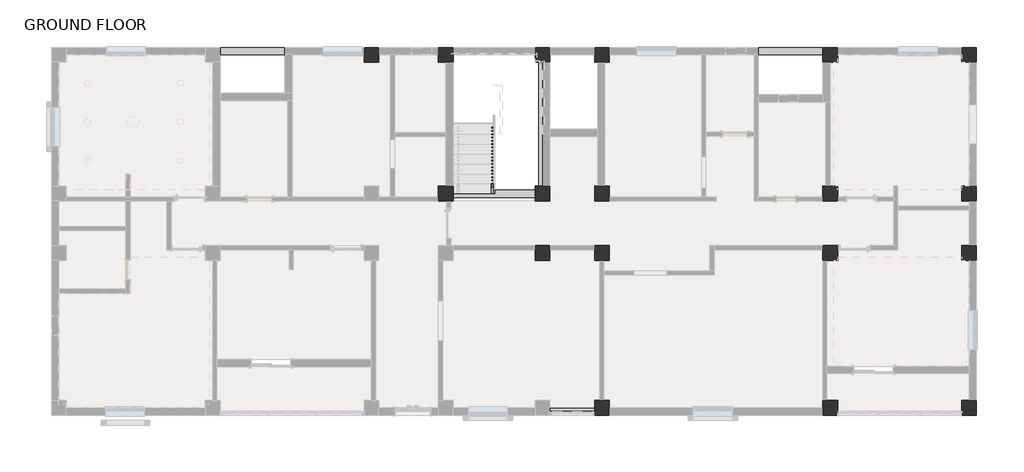
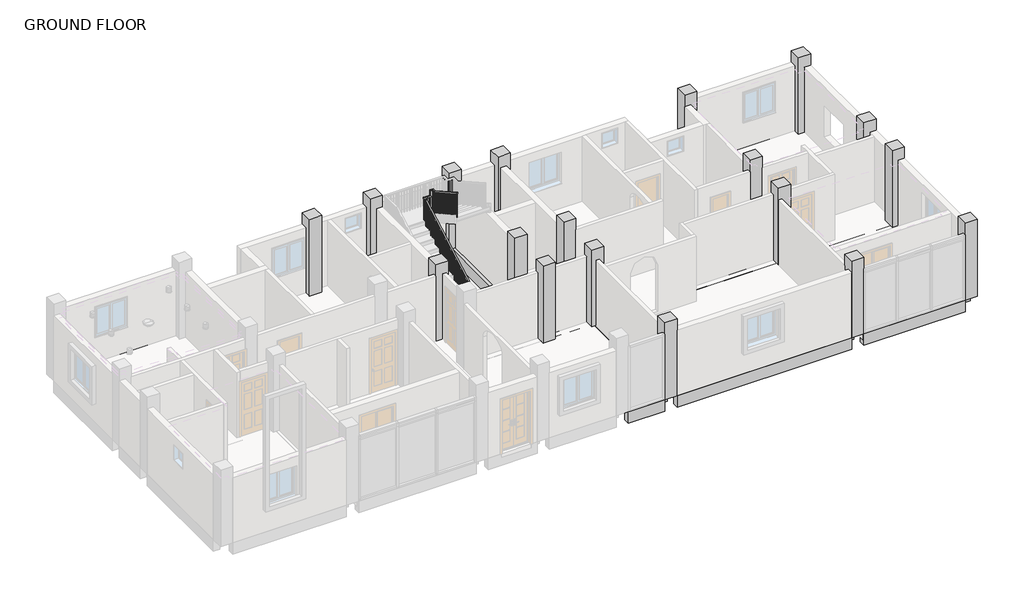
# One storey, part 4 of 5: 31 beams, 18 columns, 1 railing.
"""IFC4 building model written with IfcOpenShell, lengths in millimetres."""

from ifc_helpers import new_model, si_unit, frame, origin, place, context, project, spatial, polyline, outline, extrude, faceted_brep, element, save

model = new_model("IFC4")

# Units and contexts
model_context = context("Model", 3, world=origin())
ifc_project = project(units=[si_unit("LENGTHUNIT", "METRE", prefix="MILLI")], contexts=[model_context])

# Site, building, storey
site = spatial("IfcSite", under=ifc_project)
building = spatial("IfcBuilding", under=site)
storey = spatial("IfcBuildingStorey", under=building, Name="GROUND FLOOR", Elevation=304.8)

# Beams
placement = place(None, origin())
element("IfcBeam", 1, ObjectType="Concrete-Rectangular Beam : 9\" X 18\" BEAM", at=placement, inside=storey, context=model_context, shape_type="SweptSolid", body=[
    extrude(outline(polyline([(1310.3916602, -10887.8679047), (1310.3916602, -11116.4679047), (-61.2083398, -11116.4679047), (-61.2083398, -10887.8679047), (1310.3916602, -10887.8679047)])), frame((0.0, 0.0, -152.4), z_axis=(0.0, 0.0, 1.0), x_axis=(1.0, 0.0, 0.0)), (0.0, 0.0, 1.0), 457.2),
])
element("IfcBeam", 2, ObjectType="Concrete-Rectangular Beam : 9\" X 18\" BEAM", at=placement, inside=storey, context=model_context, shape_type="Brep", body=[
    faceted_brep([(1424.6916602, -6358.3794704, 304.8), (1424.6916602, -10659.2679047, 304.8), (1653.2916602, -10659.2679047, 304.8), (1653.2916602, -6675.8794704, 304.8), (1589.7916602, -6675.8794704, 304.8), (1589.7916602, -6358.3794704, 304.8), (1653.2916602, -10659.2679047, -152.4), (1653.2916602, -6358.3794704, -152.4), (1653.2916602, -6358.3794704, 152.4), (1653.2916602, -6675.8794704, 152.4), (1424.6916602, -10659.2679047, -152.4), (1424.6916602, -6358.3794704, -152.4), (1589.7916602, -6358.3794704, 152.4), (1589.7916602, -6675.8794704, 152.4)], [[[0, 1, 2, 3, 4, 5]], [[6, 7, 8, 9, 3, 2]], [[7, 6, 10, 11]], [[1, 0, 11, 10]], [[1, 10, 6, 2]], [[7, 11, 0, 5, 12, 8]], [[12, 13, 9, 8]], [[13, 4, 3, 9]], [[13, 12, 5, 4]]]),
])
element("IfcBeam", 3, ObjectType="Concrete-Rectangular Beam : 9\" X 18\" BEAM", at=placement, inside=storey, context=model_context, shape_type="SweptSolid", body=[
    extrude(outline(polyline([(1653.2916602, -4529.5794704), (1653.2916602, -5901.1794704), (1424.6916602, -5901.1794704), (1424.6916602, -4529.5794704), (1653.2916602, -4529.5794704)])), frame((0.0, 0.0, -152.4), z_axis=(0.0, 0.0, 1.0), x_axis=(1.0, 0.0, 0.0)), (0.0, 0.0, 1.0), 304.8),
])
element("IfcBeam", 4, ObjectType="Concrete-Rectangular Beam : 9\" X 18\" BEAM", at=placement, inside=storey, context=model_context, shape_type="SweptSolid", body=[
    extrude(outline(polyline([(8317.2128058, -10887.8679047), (8317.2128058, -11116.4679047), (1767.5916602, -11116.4679047), (1767.5916602, -10887.8679047), (8317.2128058, -10887.8679047)])), frame((0.0, 0.0, -152.4), z_axis=(0.0, 0.0, 1.0), x_axis=(1.0, 0.0, 0.0)), (0.0, 0.0, 1.0), 457.2),
])
element("IfcBeam", 5, ObjectType="Concrete-Rectangular Beam : 9\" X 18\" BEAM", at=placement, inside=storey, context=model_context, shape_type="SweptSolid", body=[
    extrude(outline(polyline([(12584.4128058, -10887.8679047), (12584.4128058, -11116.4679047), (8774.4128058, -11116.4679047), (8774.4128058, -10887.8679047), (12584.4128058, -10887.8679047)])), frame((0.0, 0.0, -152.4), z_axis=(0.0, 0.0, 1.0), x_axis=(1.0, 0.0, 0.0)), (0.0, 0.0, 1.0), 457.2),
])
element("IfcBeam", 6, ObjectType="Concrete-Rectangular Beam : 9\" X 18\" BEAM", at=placement, inside=storey, context=model_context, shape_type="SweptSolid", body=[
    extrude(outline(polyline([(12813.0128058, -6358.3794704), (13041.6128058, -6358.3794704), (13041.6128058, -10659.2679047), (12813.0128058, -10659.2679047), (12813.0128058, -6358.3794704)])), frame((0.0, 0.0, -152.4), z_axis=(0.0, 0.0, 1.0), x_axis=(1.0, 0.0, 0.0)), (0.0, 0.0, 1.0), 457.2),
])
element("IfcBeam", 7, ObjectType="Concrete-Rectangular Beam : 9\" X 18\" BEAM", at=placement, inside=storey, context=model_context, shape_type="SweptSolid", body=[
    extrude(outline(polyline([(12813.0128058, -4529.5794704), (13041.6128058, -4529.5794704), (13041.6128058, -5901.1794704), (12813.0128058, -5901.1794704), (12813.0128058, -4529.5794704)])), frame((0.0, 0.0, -152.4), z_axis=(0.0, 0.0, 1.0), x_axis=(1.0, 0.0, 0.0)), (0.0, 0.0, 1.0), 457.2),
])
element("IfcBeam", 8, ObjectType="Concrete-Rectangular Beam : 9\" X 18\" BEAM", at=placement, inside=storey, context=model_context, shape_type="SweptSolid", body=[
    extrude(outline(polyline([(12813.0128058, -262.3794704), (13041.6128058, -262.3794704), (13041.6128058, -4072.3794704), (12813.0128058, -4072.3794704), (12813.0128058, -262.3794704)])), frame((0.0, 0.0, -152.4), z_axis=(0.0, 0.0, 1.0), x_axis=(1.0, 0.0, 0.0)), (0.0, 0.0, 1.0), 457.2),
])
element("IfcBeam", 9, ObjectType="Concrete-Rectangular Beam : 9\" X 18\" BEAM", at=placement, inside=storey, context=model_context, shape_type="SweptSolid", body=[
    extrude(outline(polyline([(8774.4128058, -33.7794704), (8774.4128058, 194.8205296), (12584.4128058, 194.8205296), (12584.4128058, -33.7794704), (8774.4128058, -33.7794704)])), frame((0.0, 0.0, -152.4), z_axis=(0.0, 0.0, 1.0), x_axis=(1.0, 0.0, 0.0)), (0.0, 0.0, 1.0), 457.2),
])
element("IfcBeam", 10, ObjectType="Concrete-Rectangular Beam : 9\" X 18\" BEAM", at=placement, inside=storey, context=model_context, shape_type="SweptSolid", body=[
    extrude(outline(polyline([(1767.5916602, -33.7794704), (1767.5916602, 194.8205296), (8317.2128058, 194.8205296), (8317.2128058, -33.7794704), (1767.5916602, -33.7794704)])), frame((0.0, 0.0, -152.4), z_axis=(0.0, 0.0, 1.0), x_axis=(1.0, 0.0, 0.0)), (0.0, 0.0, 1.0), 457.2),
])
element("IfcBeam", 11, ObjectType="Concrete-Rectangular Beam : 9\" X 18\" BEAM", at=placement, inside=storey, context=model_context, shape_type="SweptSolid", body=[
    extrude(outline(polyline([(-61.2083398, -33.7794704), (-61.2083398, 194.8205296), (1310.3916602, 194.8205296), (1310.3916602, -33.7794704), (-61.2083398, -33.7794704)])), frame((0.0, 0.0, -152.4), z_axis=(0.0, 0.0, 1.0), x_axis=(1.0, 0.0, 0.0)), (0.0, 0.0, 1.0), 457.2),
])
element("IfcBeam", 12, ObjectType="Concrete-Rectangular Beam : 9\" X 18\" BEAM", at=placement, inside=storey, context=model_context, shape_type="SweptSolid", body=[
    extrude(outline(polyline([(-3029.5456086, -33.7794704), (-3029.5456086, 194.8205296), (-518.4083398, 194.8205296), (-518.4083398, -33.7794704), (-3029.5456086, -33.7794704)])), frame((0.0, 0.0, -152.4), z_axis=(0.0, 0.0, 1.0), x_axis=(1.0, 0.0, 0.0)), (0.0, 0.0, 1.0), 457.2),
])
element("IfcBeam", 13, ObjectType="Concrete-Rectangular Beam : 9\" X 18\" BEAM", at=placement, inside=storey, context=model_context, shape_type="SweptSolid", body=[
    extrude(outline(polyline([(-5315.5456086, -33.7794704), (-5315.5456086, 194.8205296), (-3486.7456086, 194.8205296), (-3486.7456086, -33.7794704), (-5315.5456086, -33.7794704)])), frame((0.0, 0.0, -152.4), z_axis=(0.0, 0.0, 1.0), x_axis=(1.0, 0.0, 0.0)), (0.0, 0.0, 1.0), 457.2),
])
element("IfcBeam", 14, ObjectType="Concrete-Rectangular Beam : 9\" X 18\" BEAM", at=placement, inside=storey, context=model_context, shape_type="SweptSolid", body=[
    extrude(outline(polyline([(-10192.3456086, -33.7794704), (-10192.3456086, 194.8205296), (-5772.7456086, 194.8205296), (-5772.7456086, -33.7794704), (-10192.3456086, -33.7794704)])), frame((0.0, 0.0, -152.4), z_axis=(0.0, 0.0, 1.0), x_axis=(1.0, 0.0, 0.0)), (0.0, 0.0, 1.0), 457.2),
])
element("IfcBeam", 15, ObjectType="Concrete-Rectangular Beam : 9\" X 18\" BEAM", at=placement, inside=storey, context=model_context, shape_type="SweptSolid", body=[
    extrude(outline(polyline([(-14916.7456086, -33.7794704), (-14916.7456086, 194.8205296), (-10649.5456086, 194.8205296), (-10649.5456086, -33.7794704), (-14916.7456086, -33.7794704)])), frame((0.0, 0.0, -152.4), z_axis=(0.0, 0.0, 1.0), x_axis=(1.0, 0.0, 0.0)), (0.0, 0.0, 1.0), 457.2),
])
element("IfcBeam", 16, ObjectType="Concrete-Rectangular Beam : 9\" X 18\" BEAM", at=placement, inside=storey, context=model_context, shape_type="SweptSolid", body=[
    extrude(outline(polyline([(-518.4083398, -4186.6794704), (-518.4083398, -4415.2794704), (-3029.5456086, -4415.2794704), (-3029.5456086, -4186.6794704), (-518.4083398, -4186.6794704)])), frame((0.0, 0.0, -152.4), z_axis=(0.0, 0.0, 1.0), x_axis=(1.0, 0.0, 0.0)), (0.0, 0.0, 1.0), 457.2),
])
element("IfcBeam", 17, ObjectType="Concrete-Rectangular Beam : 9\" X 18\" BEAM", at=placement, inside=storey, context=model_context, shape_type="SweptSolid", body=[
    extrude(outline(polyline([(1310.3916602, -4415.2794704), (-61.2083398, -4415.2794704), (-61.2083398, -4186.6794704), (1310.3916602, -4186.6794704), (1310.3916602, -4415.2794704)])), frame((0.0, 0.0, -152.4), z_axis=(0.0, 0.0, 1.0), x_axis=(1.0, 0.0, 0.0)), (0.0, 0.0, 1.0), 304.8),
])
element("IfcBeam", 18, ObjectType="Concrete-Rectangular Beam : 9\" X 18\" BEAM", at=placement, inside=storey, context=model_context, shape_type="SweptSolid", body=[
    extrude(outline(polyline([(1424.6916602, -262.3794704), (1653.2916602, -262.3794704), (1653.2916602, -4072.3794704), (1424.6916602, -4072.3794704), (1424.6916602, -262.3794704)])), frame((0.0, 0.0, -152.4), z_axis=(0.0, 0.0, 1.0), x_axis=(1.0, 0.0, 0.0)), (0.0, 0.0, 1.0), 457.2),
])
element("IfcBeam", 19, ObjectType="Concrete-Rectangular Beam : 9\" X 18\" BEAM", at=placement, inside=storey, context=model_context, shape_type="SweptSolid", body=[
    extrude(outline(polyline([(-175.5083398, -4072.3794704), (-404.1083398, -4072.3794704), (-404.1083398, -262.3794704), (-175.5083398, -262.3794704), (-175.5083398, -4072.3794704)])), frame((0.0, 0.0, -152.4), z_axis=(0.0, 0.0, 1.0), x_axis=(1.0, 0.0, 0.0)), (0.0, 0.0, 1.0), 457.2),
])
element("IfcBeam", 20, ObjectType="Concrete-Rectangular Beam : 9\" X 18\" BEAM", at=placement, inside=storey, context=model_context, shape_type="SweptSolid", body=[
    extrude(outline(polyline([(-3143.8456086, -4072.3794704), (-3372.4456086, -4072.3794704), (-3372.4456086, -262.3794704), (-3143.8456086, -262.3794704), (-3143.8456086, -4072.3794704)])), frame((0.0, 0.0, -152.4), z_axis=(0.0, 0.0, 1.0), x_axis=(1.0, 0.0, 0.0)), (0.0, 0.0, 1.0), 457.2),
])
element("IfcBeam", 21, ObjectType="Concrete-Rectangular Beam : 9\" X 18\" BEAM", at=placement, inside=storey, context=model_context, shape_type="SweptSolid", body=[
    extrude(outline(polyline([(-5429.8456086, -4072.3794704), (-5658.4456086, -4072.3794704), (-5658.4456086, -262.3794704), (-5429.8456086, -262.3794704), (-5429.8456086, -4072.3794704)])), frame((0.0, 0.0, -152.4), z_axis=(0.0, 0.0, 1.0), x_axis=(1.0, 0.0, 0.0)), (0.0, 0.0, 1.0), 457.2),
])
element("IfcBeam", 22, ObjectType="Concrete-Rectangular Beam : 9\" X 18\" BEAM", at=placement, inside=storey, context=model_context, shape_type="SweptSolid", body=[
    extrude(outline(polyline([(1310.3916602, -6015.4794704), (1310.3916602, -6244.0794704), (-61.2083398, -6244.0794704), (-61.2083398, -6015.4794704), (1310.3916602, -6015.4794704)])), frame((0.0, 0.0, -152.4), z_axis=(0.0, 0.0, 1.0), x_axis=(1.0, 0.0, 0.0)), (0.0, 0.0, 1.0), 457.2),
])
element("IfcBeam", 23, ObjectType="Concrete-Rectangular Beam : 9\" X 18\" BEAM", at=placement, inside=storey, context=model_context, shape_type="SweptSolid", body=[
    extrude(outline(polyline([(-175.5083398, -4529.5794704), (-175.5083398, -5901.1794704), (-404.1083398, -5901.1794704), (-404.1083398, -4529.5794704), (-175.5083398, -4529.5794704)])), frame((0.0, 0.0, -152.4), z_axis=(0.0, 0.0, 1.0), x_axis=(1.0, 0.0, 0.0)), (0.0, 0.0, 1.0), 304.8),
])
element("IfcBeam", 24, ObjectType="Concrete-Rectangular Beam : 9\" X 18\" BEAM", at=placement, inside=storey, context=model_context, shape_type="Brep", body=[
    faceted_brep([(-3232.7456086, -5901.1794704, 304.8), (-3143.8456086, -5901.1794704, 304.8), (-3143.8456086, -5672.5794704, 304.8), (-3232.7456086, -5672.5794704, 304.8), (-3372.4456086, -4529.5794704, -152.4), (-3372.4456086, -5901.1794704, -152.4), (-3372.4456086, -5901.1794704, 152.4), (-3372.4456086, -4529.5794704, 152.4), (-3143.8456086, -4529.5794704, -152.4), (-3143.8456086, -5901.1794704, -152.4), (-3143.8456086, -4529.5794704, 152.4), (-3143.8456086, -5672.5794704, 152.4), (-3232.7456086, -5901.1794704, 152.4), (-3232.7456086, -5672.5794704, 152.4)], [[[0, 1, 2, 3]], [[4, 5, 6, 7]], [[5, 4, 8, 9]], [[9, 8, 10, 11, 2, 1]], [[8, 4, 7, 10]], [[5, 9, 1, 0, 12, 6]], [[12, 13, 11, 10, 7, 6]], [[13, 3, 2, 11]], [[13, 12, 0, 3]]]),
])
element("IfcBeam", 25, ObjectType="Concrete-Rectangular Beam : 9\" X 18\" BEAM", at=placement, inside=storey, context=model_context, shape_type="Brep", body=[
    faceted_brep([(1767.5916602, -4186.6794704, 304.8), (1767.5916602, -4415.2794704, 304.8), (5044.1916602, -4415.2794704, 304.8), (5044.1916602, -4402.5794704, 304.8), (4726.6916602, -4402.5794704, 304.8), (4726.6916602, -4186.6794704, 304.8), (1767.5916602, -4415.2794704, -152.4), (8317.2128058, -4415.2794704, -152.4), (8317.2128058, -4415.2794704, 304.8), (6212.5916602, -4415.2794704, 304.8), (6212.5916602, -4415.2794704, 152.4), (5044.1916602, -4415.2794704, 152.4), (1767.5916602, -4186.6794704, -152.4), (8317.2128058, -4186.6794704, -152.4), (4726.6916602, -4186.6794704, 152.4), (6212.5916602, -4186.6794704, 152.4), (6212.5916602, -4186.6794704, 304.8), (8317.2128058, -4186.6794704, 304.8), (4726.6916602, -4402.5794704, 152.4), (5044.1916602, -4402.5794704, 152.4)], [[[0, 1, 2, 3, 4, 5]], [[6, 7, 8, 9, 10, 11, 2, 1]], [[7, 6, 12, 13]], [[13, 12, 0, 5, 14, 15, 16, 17]], [[0, 12, 6, 1]], [[17, 8, 7, 13]], [[18, 19, 11, 10, 15, 14]], [[19, 3, 2, 11]], [[19, 18, 4, 3]], [[4, 18, 14, 5]], [[15, 10, 9, 16]], [[8, 17, 16, 9]]]),
])
element("IfcBeam", 26, ObjectType="Concrete-Rectangular Beam : 9\" X 18\" BEAM", at=placement, inside=storey, context=model_context, shape_type="SweptSolid", body=[
    extrude(outline(polyline([(12584.4128058, -4186.6794704), (12584.4128058, -4415.2794704), (8774.4128058, -4415.2794704), (8774.4128058, -4186.6794704), (12584.4128058, -4186.6794704)])), frame((0.0, 0.0, -152.4), z_axis=(0.0, 0.0, 1.0), x_axis=(1.0, 0.0, 0.0)), (0.0, 0.0, 1.0), 457.2),
])
element("IfcBeam", 27, ObjectType="Concrete-Rectangular Beam : 9\" X 18\" BEAM", at=placement, inside=storey, context=model_context, shape_type="SweptSolid", body=[
    extrude(outline(polyline([(8774.4128058, -6244.0794704), (8774.4128058, -6015.4794704), (12584.4128058, -6015.4794704), (12584.4128058, -6244.0794704), (8774.4128058, -6244.0794704)])), frame((0.0, 0.0, -152.4), z_axis=(0.0, 0.0, 1.0), x_axis=(1.0, 0.0, 0.0)), (0.0, 0.0, 1.0), 457.2),
])
element("IfcBeam", 28, ObjectType="Concrete-Rectangular Beam : 9\" X 18\" BEAM", at=placement, inside=storey, context=model_context, shape_type="SweptSolid", body=[
    extrude(outline(polyline([(-152.4, 1767.5916602), (-152.4, 8317.2128058), (304.8, 8317.2128058), (304.8, 4853.6916602), (152.4, 4853.6916602), (152.4, 1767.5916602), (-152.4, 1767.5916602)])), frame((0.0, -6244.0794704, 0.0), z_axis=(0.0, 1.0, 0.0), x_axis=(0.0, 0.0, 1.0)), (0.0, 0.0, 1.0), 228.6),
])
element("IfcBeam", 29, ObjectType="Concrete-Rectangular Beam : 9\" X 18\" BEAM", at=placement, inside=storey, context=model_context, shape_type="SweptSolid", body=[
    extrude(outline(polyline([(8431.5128058, -6358.3794704), (8660.1128058, -6358.3794704), (8660.1128058, -10659.2679047), (8431.5128058, -10659.2679047), (8431.5128058, -6358.3794704)])), frame((0.0, 0.0, -152.4), z_axis=(0.0, 0.0, 1.0), x_axis=(1.0, 0.0, 0.0)), (0.0, 0.0, 1.0), 457.2),
])
element("IfcBeam", 30, ObjectType="Concrete-Rectangular Beam : 9\" X 18\" BEAM", at=placement, inside=storey, context=model_context, shape_type="SweptSolid", body=[
    extrude(outline(polyline([(8660.1128058, -4529.5794704), (8660.1128058, -5901.1794704), (8431.5128058, -5901.1794704), (8431.5128058, -4529.5794704), (8660.1128058, -4529.5794704)])), frame((0.0, 0.0, -152.4), z_axis=(0.0, 0.0, 1.0), x_axis=(1.0, 0.0, 0.0)), (0.0, 0.0, 1.0), 304.8),
])
element("IfcBeam", 31, ObjectType="Concrete-Rectangular Beam : 9\" X 18\" BEAM", at=placement, inside=storey, context=model_context, shape_type="SweptSolid", body=[
    extrude(outline(polyline([(8431.5128058, -262.3794704), (8660.1128058, -262.3794704), (8660.1128058, -4072.3794704), (8431.5128058, -4072.3794704), (8431.5128058, -262.3794704)])), frame((0.0, 0.0, -152.4), z_axis=(0.0, 0.0, 1.0), x_axis=(1.0, 0.0, 0.0)), (0.0, 0.0, 1.0), 457.2),
])

# Columns
element("IfcColumn", 32, ObjectType="Concrete-Rectangular-Column : COLUMN 18\" X 18\"", at=placement, inside=storey, context=model_context, shape_type="SweptSolid", body=[
    extrude(outline(polyline([(-5315.5456086, 194.8205296), (-5315.5456086, -262.3794704), (-5772.7456086, -262.3794704), (-5772.7456086, 194.8205296), (-5315.5456086, 194.8205296)])), frame((0.0, 0.0, 304.8), z_axis=(0.0, 0.0, 1.0), x_axis=(1.0, 0.0, 0.0)), (0.0, 0.0, 1.0), 3048.0),
])
element("IfcColumn", 33, ObjectType="Concrete-Rectangular-Column : COLUMN 18\" X 18\"", at=placement, inside=storey, context=model_context, shape_type="SweptSolid", body=[
    extrude(outline(polyline([(-3029.5456086, 194.8205296), (-3029.5456086, -262.3794704), (-3486.7456086, -262.3794704), (-3486.7456086, 194.8205296), (-3029.5456086, 194.8205296)])), frame((0.0, 0.0, 304.8), z_axis=(0.0, 0.0, 1.0), x_axis=(1.0, 0.0, 0.0)), (0.0, 0.0, 1.0), 3048.0),
])
element("IfcColumn", 34, ObjectType="Concrete-Rectangular-Column : COLUMN 18\" X 18\"", at=placement, inside=storey, context=model_context, shape_type="SweptSolid", body=[
    extrude(outline(polyline([(-61.2083398, 194.8205296), (-61.2083398, -262.3794704), (-518.4083398, -262.3794704), (-518.4083398, 194.8205296), (-61.2083398, 194.8205296)])), frame((0.0, 0.0, 304.8), z_axis=(0.0, 0.0, 1.0), x_axis=(1.0, 0.0, 0.0)), (0.0, 0.0, 1.0), 3048.0),
])
element("IfcColumn", 35, ObjectType="Concrete-Rectangular-Column : COLUMN 18\" X 18\"", at=placement, inside=storey, context=model_context, shape_type="SweptSolid", body=[
    extrude(outline(polyline([(1767.5916602, 194.8205296), (1767.5916602, -262.3794704), (1310.3916602, -262.3794704), (1310.3916602, 194.8205296), (1767.5916602, 194.8205296)])), frame((0.0, 0.0, 304.8), z_axis=(0.0, 0.0, 1.0), x_axis=(1.0, 0.0, 0.0)), (0.0, 0.0, 1.0), 3048.0),
])
element("IfcColumn", 36, ObjectType="Concrete-Rectangular-Column : COLUMN 18\" X 18\"", at=placement, inside=storey, context=model_context, shape_type="SweptSolid", body=[
    extrude(outline(polyline([(8774.4128058, 194.8205296), (8774.4128058, -262.3794704), (8317.2128058, -262.3794704), (8317.2128058, 194.8205296), (8774.4128058, 194.8205296)])), frame((0.0, 0.0, 304.8), z_axis=(0.0, 0.0, 1.0), x_axis=(1.0, 0.0, 0.0)), (0.0, 0.0, 1.0), 3048.0),
])
element("IfcColumn", 37, ObjectType="Concrete-Rectangular-Column : COLUMN 18\" X 18\"", at=placement, inside=storey, context=model_context, shape_type="SweptSolid", body=[
    extrude(outline(polyline([(13041.6128058, 194.8205296), (13041.6128058, -262.3794704), (12584.4128058, -262.3794704), (12584.4128058, 194.8205296), (13041.6128058, 194.8205296)])), frame((0.0, 0.0, 304.8), z_axis=(0.0, 0.0, 1.0), x_axis=(1.0, 0.0, 0.0)), (0.0, 0.0, 1.0), 3048.0),
])
element("IfcColumn", 38, ObjectType="Concrete-Rectangular-Column : COLUMN 18\" X 18\"", at=placement, inside=storey, context=model_context, shape_type="SweptSolid", body=[
    extrude(outline(polyline([(13041.6128058, -4072.3794704), (13041.6128058, -4529.5794704), (12584.4128058, -4529.5794704), (12584.4128058, -4072.3794704), (13041.6128058, -4072.3794704)])), frame((0.0, 0.0, 304.8), z_axis=(0.0, 0.0, 1.0), x_axis=(1.0, 0.0, 0.0)), (0.0, 0.0, 1.0), 3048.0),
])
element("IfcColumn", 39, ObjectType="Concrete-Rectangular-Column : COLUMN 18\" X 18\"", at=placement, inside=storey, context=model_context, shape_type="SweptSolid", body=[
    extrude(outline(polyline([(13041.6128058, -5901.1794704), (13041.6128058, -6358.3794704), (12584.4128058, -6358.3794704), (12584.4128058, -5901.1794704), (13041.6128058, -5901.1794704)])), frame((0.0, 0.0, 304.8), z_axis=(0.0, 0.0, 1.0), x_axis=(1.0, 0.0, 0.0)), (0.0, 0.0, 1.0), 3048.0),
])
element("IfcColumn", 40, ObjectType="Concrete-Rectangular-Column : COLUMN 18\" X 18\"", at=placement, inside=storey, context=model_context, shape_type="SweptSolid", body=[
    extrude(outline(polyline([(13041.6128058, -10659.2679047), (13041.6128058, -11116.4679047), (12584.4128058, -11116.4679047), (12584.4128058, -10659.2679047), (13041.6128058, -10659.2679047)])), frame((0.0, 0.0, 304.8), z_axis=(0.0, 0.0, 1.0), x_axis=(1.0, 0.0, 0.0)), (0.0, 0.0, 1.0), 3048.0),
])
element("IfcColumn", 41, ObjectType="Concrete-Rectangular-Column : COLUMN 18\" X 18\"", at=placement, inside=storey, context=model_context, shape_type="SweptSolid", body=[
    extrude(outline(polyline([(8774.4128058, -10659.2679047), (8774.4128058, -11116.4679047), (8317.2128058, -11116.4679047), (8317.2128058, -10659.2679047), (8774.4128058, -10659.2679047)])), frame((0.0, 0.0, 304.8), z_axis=(0.0, 0.0, 1.0), x_axis=(1.0, 0.0, 0.0)), (0.0, 0.0, 1.0), 3048.0),
])
element("IfcColumn", 42, ObjectType="Concrete-Rectangular-Column : COLUMN 18\" X 18\"", at=placement, inside=storey, context=model_context, shape_type="SweptSolid", body=[
    extrude(outline(polyline([(1767.5916602, -10659.2679047), (1767.5916602, -11116.4679047), (1310.3916602, -11116.4679047), (1310.3916602, -10659.2679047), (1767.5916602, -10659.2679047)])), frame((0.0, 0.0, 304.8), z_axis=(0.0, 0.0, 1.0), x_axis=(1.0, 0.0, 0.0)), (0.0, 0.0, 1.0), 3048.0),
])
element("IfcColumn", 43, ObjectType="Concrete-Rectangular-Column : COLUMN 18\" X 18\"", at=placement, inside=storey, context=model_context, shape_type="SweptSolid", body=[
    extrude(outline(polyline([(-3029.5456086, -4072.3794704), (-3029.5456086, -4529.5794704), (-3486.7456086, -4529.5794704), (-3486.7456086, -4072.3794704), (-3029.5456086, -4072.3794704)])), frame((0.0, 0.0, 304.8), z_axis=(0.0, 0.0, 1.0), x_axis=(1.0, 0.0, 0.0)), (0.0, 0.0, 1.0), 3048.0),
])
element("IfcColumn", 44, ObjectType="Concrete-Rectangular-Column : COLUMN 18\" X 18\"", at=placement, inside=storey, context=model_context, shape_type="SweptSolid", body=[
    extrude(outline(polyline([(-61.2083398, -4072.3794704), (-61.2083398, -4529.5794704), (-518.4083398, -4529.5794704), (-518.4083398, -4072.3794704), (-61.2083398, -4072.3794704)])), frame((0.0, 0.0, 304.8), z_axis=(0.0, 0.0, 1.0), x_axis=(1.0, 0.0, 0.0)), (0.0, 0.0, 1.0), 3048.0),
])
element("IfcColumn", 45, ObjectType="Concrete-Rectangular-Column : COLUMN 18\" X 18\"", at=placement, inside=storey, context=model_context, shape_type="SweptSolid", body=[
    extrude(outline(polyline([(1767.5916602, -4072.3794704), (1767.5916602, -4529.5794704), (1310.3916602, -4529.5794704), (1310.3916602, -4072.3794704), (1767.5916602, -4072.3794704)])), frame((0.0, 0.0, 304.8), z_axis=(0.0, 0.0, 1.0), x_axis=(1.0, 0.0, 0.0)), (0.0, 0.0, 1.0), 3048.0),
])
element("IfcColumn", 46, ObjectType="Concrete-Rectangular-Column : COLUMN 18\" X 18\"", at=placement, inside=storey, context=model_context, shape_type="SweptSolid", body=[
    extrude(outline(polyline([(8774.4128058, -4072.3794704), (8774.4128058, -4529.5794704), (8317.2128058, -4529.5794704), (8317.2128058, -4072.3794704), (8774.4128058, -4072.3794704)])), frame((0.0, 0.0, 304.8), z_axis=(0.0, 0.0, 1.0), x_axis=(1.0, 0.0, 0.0)), (0.0, 0.0, 1.0), 3048.0),
])
element("IfcColumn", 47, ObjectType="Concrete-Rectangular-Column : COLUMN 18\" X 18\"", at=placement, inside=storey, context=model_context, shape_type="SweptSolid", body=[
    extrude(outline(polyline([(8774.4128058, -5901.1794704), (8774.4128058, -6358.3794704), (8317.2128058, -6358.3794704), (8317.2128058, -5901.1794704), (8774.4128058, -5901.1794704)])), frame((0.0, 0.0, 304.8), z_axis=(0.0, 0.0, 1.0), x_axis=(1.0, 0.0, 0.0)), (0.0, 0.0, 1.0), 3048.0),
])
element("IfcColumn", 48, ObjectType="Concrete-Rectangular-Column : COLUMN 18\" X 18\"", at=placement, inside=storey, context=model_context, shape_type="SweptSolid", body=[
    extrude(outline(polyline([(1767.5916602, -5901.1794704), (1767.5916602, -6358.3794704), (1310.3916602, -6358.3794704), (1310.3916602, -5901.1794704), (1767.5916602, -5901.1794704)])), frame((0.0, 0.0, 304.8), z_axis=(0.0, 0.0, 1.0), x_axis=(1.0, 0.0, 0.0)), (0.0, 0.0, 1.0), 3048.0),
])
element("IfcColumn", 49, ObjectType="Concrete-Rectangular-Column : COLUMN 18\" X 18\"", at=placement, inside=storey, context=model_context, shape_type="SweptSolid", body=[
    extrude(outline(polyline([(-61.2083398, -5901.1794704), (-61.2083398, -6358.3794704), (-518.4083398, -6358.3794704), (-518.4083398, -5901.1794704), (-61.2083398, -5901.1794704)])), frame((0.0, 0.0, 304.8), z_axis=(0.0, 0.0, 1.0), x_axis=(1.0, 0.0, 0.0)), (0.0, 0.0, 1.0), 3048.0),
])

# Railing
element("IfcRailing", 50, ObjectType="Handrail - Rectangular", at=placement, inside=storey, context=model_context, shape_type="SolidModel", body=[
    faceted_brep([(-1861.1456086, -4300.9794704, 1388.5333333), (-1861.1456086, -4300.9794704, 1330.420221), (-1810.3456086, -4300.9794704, 1330.420221), (-1810.3456086, -4300.9794704, 1388.5333333), (-1861.1456086, -1024.3794704, 3208.8666667), (-1861.1456086, -973.5794704, 3178.9757765), (-1810.3456086, -973.5794704, 3178.9757765), (-1810.3456086, -1024.3794704, 3208.8666667), (-1861.1456086, -1024.3794704, 3251.2), (-1861.1456086, -973.5794704, 3200.4), (-1810.3456086, -973.5794704, 3200.4), (-1810.3456086, -1024.3794704, 3251.2), (-1861.1456086, -897.3794704, 3251.2), (-1861.1456086, -897.3794704, 3200.4), (-1810.3456086, -948.1794704, 3200.4), (-1810.3456086, -948.1794704, 3251.2), (-1734.1456086, -897.3794704, 3251.2), (-1734.1456086, -897.3794704, 3200.4), (-1734.1456086, -948.1794704, 3200.4), (-1734.1456086, -948.1794704, 3251.2), (-1610.6083398, -897.3794704, 3251.2), (-1559.8083398, -897.3794704, 3200.4), (-1559.8083398, -948.1794704, 3200.4), (-1610.6083398, -948.1794704, 3251.2), (-1610.6083398, -897.3794704, 3462.8666667), (-1559.8083398, -897.3794704, 3412.0666667), (-1559.8083398, -948.1794704, 3412.0666667), (-1610.6083398, -948.1794704, 3462.8666667), (-1483.6083398, -897.3794704, 3462.8666667), (-1483.6083398, -897.3794704, 3412.0666667), (-1534.4083398, -948.1794704, 3412.0666667), (-1534.4083398, -948.1794704, 3462.8666667), (-1483.6083398, -1024.3794704, 3462.8666667), (-1483.6083398, -1037.5430727, 3412.0666667), (-1534.4083398, -1037.5430727, 3412.0666667), (-1534.4083398, -1024.3794704, 3462.8666667), (-1483.6083398, -2472.1794704, 4267.2), (-1534.4083398, -2472.1794704, 4267.2), (-1534.4083398, -2472.1794704, 4209.0868876), (-1483.6083398, -2472.1794704, 4209.0868876)], [[[0, 1, 2, 3]], [[1, 0, 4, 5]], [[2, 1, 5, 6]], [[3, 2, 6, 7]], [[0, 3, 7, 4]], [[5, 4, 8, 9]], [[6, 5, 9, 10]], [[7, 6, 10, 11]], [[4, 7, 11, 8]], [[9, 8, 12, 13]], [[10, 9, 13, 14]], [[11, 10, 14, 15]], [[8, 11, 15, 12]], [[13, 12, 16, 17]], [[14, 13, 17, 18]], [[15, 14, 18, 19]], [[12, 15, 19, 16]], [[17, 16, 20, 21]], [[18, 17, 21, 22]], [[19, 18, 22, 23]], [[16, 19, 23, 20]], [[21, 20, 24, 25]], [[22, 21, 25, 26]], [[23, 22, 26, 27]], [[20, 23, 27, 24]], [[25, 24, 28, 29]], [[26, 25, 29, 30]], [[27, 26, 30, 31]], [[24, 27, 31, 28]], [[29, 28, 32, 33]], [[30, 29, 33, 34]], [[31, 30, 34, 35]], [[28, 31, 35, 32]], [[36, 37, 38, 39]], [[33, 32, 36, 39]], [[34, 33, 39, 38]], [[35, 34, 38, 37]], [[32, 35, 37, 36]]]),
    extrude(outline(polyline([(-2456.3044704, 4200.2674432), (-2437.2544704, 4189.6841099), (-2437.2544704, 3183.4666667), (-2456.3044704, 3183.4666667), (-2456.3044704, 4200.2674432)])), frame((-1518.5333398, 0.0, 0.0), z_axis=(1.0, 0.0, 0.0), x_axis=(0.0, 1.0, 0.0)), (0.0, 0.0, 1.0), 19.05),
    extrude(outline(polyline([(-2354.7044704, 4143.8229988), (-2335.6544704, 4133.2396654), (-2335.6544704, 3183.4666667), (-2354.7044704, 3183.4666667), (-2354.7044704, 4143.8229988)])), frame((-1518.5333398, 0.0, 0.0), z_axis=(1.0, 0.0, 0.0), x_axis=(0.0, 1.0, 0.0)), (0.0, 0.0, 1.0), 19.05),
    extrude(outline(polyline([(-2253.1044704, 4087.3785543), (-2234.0544704, 4076.795221), (-2234.0544704, 3183.4666667), (-2253.1044704, 3183.4666667), (-2253.1044704, 4087.3785543)])), frame((-1518.5333398, 0.0, 0.0), z_axis=(1.0, 0.0, 0.0), x_axis=(0.0, 1.0, 0.0)), (0.0, 0.0, 1.0), 19.05),
    extrude(outline(polyline([(-2151.5044704, 4030.9341099), (-2132.4544704, 4020.3507765), (-2132.4544704, 3014.1333333), (-2151.5044704, 3014.1333333), (-2151.5044704, 4030.9341099)])), frame((-1518.5333398, 0.0, 0.0), z_axis=(1.0, 0.0, 0.0), x_axis=(0.0, 1.0, 0.0)), (0.0, 0.0, 1.0), 19.05),
    extrude(outline(polyline([(-2049.9044704, 3974.4896654), (-2030.8544704, 3963.9063321), (-2030.8544704, 3014.1333333), (-2049.9044704, 3014.1333333), (-2049.9044704, 3974.4896654)])), frame((-1518.5333398, 0.0, 0.0), z_axis=(1.0, 0.0, 0.0), x_axis=(0.0, 1.0, 0.0)), (0.0, 0.0, 1.0), 19.05),
    extrude(outline(polyline([(-1948.3044704, 3918.045221), (-1929.2544704, 3907.4618876), (-1929.2544704, 3014.1333333), (-1948.3044704, 3014.1333333), (-1948.3044704, 3918.045221)])), frame((-1518.5333398, 0.0, 0.0), z_axis=(1.0, 0.0, 0.0), x_axis=(0.0, 1.0, 0.0)), (0.0, 0.0, 1.0), 19.05),
    extrude(outline(polyline([(-1846.7044704, 3861.6007765), (-1827.6544704, 3851.0174432), (-1827.6544704, 2844.8), (-1846.7044704, 2844.8), (-1846.7044704, 3861.6007765)])), frame((-1518.5333398, 0.0, 0.0), z_axis=(1.0, 0.0, 0.0), x_axis=(0.0, 1.0, 0.0)), (0.0, 0.0, 1.0), 19.05),
    extrude(outline(polyline([(-1745.1044704, 3805.1563321), (-1726.0544704, 3794.5729988), (-1726.0544704, 2844.8), (-1745.1044704, 2844.8), (-1745.1044704, 3805.1563321)])), frame((-1518.5333398, 0.0, 0.0), z_axis=(1.0, 0.0, 0.0), x_axis=(0.0, 1.0, 0.0)), (0.0, 0.0, 1.0), 19.05),
    extrude(outline(polyline([(-1643.5044704, 3748.7118876), (-1624.4544704, 3738.1285543), (-1624.4544704, 2844.8), (-1643.5044704, 2844.8), (-1643.5044704, 3748.7118876)])), frame((-1518.5333398, 0.0, 0.0), z_axis=(1.0, 0.0, 0.0), x_axis=(0.0, 1.0, 0.0)), (0.0, 0.0, 1.0), 19.05),
    extrude(outline(polyline([(-1541.9044704, 3692.2674432), (-1522.8544704, 3681.6841099), (-1522.8544704, 2675.4666667), (-1541.9044704, 2675.4666667), (-1541.9044704, 3692.2674432)])), frame((-1518.5333398, 0.0, 0.0), z_axis=(1.0, 0.0, 0.0), x_axis=(0.0, 1.0, 0.0)), (0.0, 0.0, 1.0), 19.05),
    extrude(outline(polyline([(-1440.3044704, 3635.8229988), (-1421.2544704, 3625.2396654), (-1421.2544704, 2675.4666667), (-1440.3044704, 2675.4666667), (-1440.3044704, 3635.8229988)])), frame((-1518.5333398, 0.0, 0.0), z_axis=(1.0, 0.0, 0.0), x_axis=(0.0, 1.0, 0.0)), (0.0, 0.0, 1.0), 19.05),
    extrude(outline(polyline([(-1338.7044704, 3579.3785543), (-1319.6544704, 3568.795221), (-1319.6544704, 2675.4666667), (-1338.7044704, 2675.4666667), (-1338.7044704, 3579.3785543)])), frame((-1518.5333398, 0.0, 0.0), z_axis=(1.0, 0.0, 0.0), x_axis=(0.0, 1.0, 0.0)), (0.0, 0.0, 1.0), 19.05),
    extrude(outline(polyline([(-1237.1044704, 3522.9341099), (-1218.0544704, 3512.3507765), (-1218.0544704, 2506.1333333), (-1237.1044704, 2506.1333333), (-1237.1044704, 3522.9341099)])), frame((-1518.5333398, 0.0, 0.0), z_axis=(1.0, 0.0, 0.0), x_axis=(0.0, 1.0, 0.0)), (0.0, 0.0, 1.0), 19.05),
    extrude(outline(polyline([(-1135.5044704, 3466.4896654), (-1116.4544704, 3455.9063321), (-1116.4544704, 2506.1333333), (-1135.5044704, 2506.1333333), (-1135.5044704, 3466.4896654)])), frame((-1518.5333398, 0.0, 0.0), z_axis=(1.0, 0.0, 0.0), x_axis=(0.0, 1.0, 0.0)), (0.0, 0.0, 1.0), 19.05),
    extrude(outline(polyline([(-1033.9044704, 3410.045221), (-1014.8544704, 3399.4618876), (-1014.8544704, 2506.1333333), (-1033.9044704, 2506.1333333), (-1033.9044704, 3410.045221)])), frame((-1518.5333398, 0.0, 0.0), z_axis=(1.0, 0.0, 0.0), x_axis=(0.0, 1.0, 0.0)), (0.0, 0.0, 1.0), 19.05),
    extrude(outline(polyline([(-1540.4706086, -932.3044704), (-1540.4706086, -913.2544704), (-1521.4206086, -913.2544704), (-1521.4206086, -932.3044704), (-1540.4706086, -932.3044704)])), frame((0.0, 0.0, 2336.8), z_axis=(0.0, 0.0, 1.0), x_axis=(1.0, 0.0, 0.0)), (0.0, 0.0, 1.0), 1075.2666667),
    extrude(outline(polyline([(-1642.0706086, -932.3044704), (-1642.0706086, -913.2544704), (-1623.0206086, -913.2544704), (-1623.0206086, -932.3044704), (-1642.0706086, -932.3044704)])), frame((0.0, 0.0, 2336.8), z_axis=(0.0, 0.0, 1.0), x_axis=(1.0, 0.0, 0.0)), (0.0, 0.0, 1.0), 863.6),
    extrude(outline(polyline([(-1743.6706086, -932.3044704), (-1743.6706086, -913.2544704), (-1724.6206086, -913.2544704), (-1724.6206086, -932.3044704), (-1743.6706086, -932.3044704)])), frame((0.0, 0.0, 2336.8), z_axis=(0.0, 0.0, 1.0), x_axis=(1.0, 0.0, 0.0)), (0.0, 0.0, 1.0), 863.6),
    extrude(outline(polyline([(-1826.2206086, -957.7044704), (-1845.2706086, -957.7044704), (-1845.2706086, -938.6544704), (-1826.2206086, -938.6544704), (-1826.2206086, -957.7044704)])), frame((0.0, 0.0, 2336.8), z_axis=(0.0, 0.0, 1.0), x_axis=(1.0, 0.0, 0.0)), (0.0, 0.0, 1.0), 863.6),
    extrude(outline(polyline([(-1059.3044704, 3131.3507765), (-1040.2544704, 3141.9341099), (-1040.2544704, 2167.4666667), (-1059.3044704, 2167.4666667), (-1059.3044704, 3131.3507765)])), frame((-1845.2706086, 0.0, 0.0), z_axis=(1.0, 0.0, 0.0), x_axis=(0.0, 1.0, 0.0)), (0.0, 0.0, 1.0), 19.05),
    extrude(outline(polyline([(-1160.9044704, 3074.9063321), (-1141.8544704, 3085.4896654), (-1141.8544704, 2167.4666667), (-1160.9044704, 2167.4666667), (-1160.9044704, 3074.9063321)])), frame((-1845.2706086, 0.0, 0.0), z_axis=(1.0, 0.0, 0.0), x_axis=(0.0, 1.0, 0.0)), (0.0, 0.0, 1.0), 19.05),
    extrude(outline(polyline([(-1262.5044704, 3018.4618876), (-1243.4544704, 3029.045221), (-1243.4544704, 2167.4666667), (-1262.5044704, 2167.4666667), (-1262.5044704, 3018.4618876)])), frame((-1845.2706086, 0.0, 0.0), z_axis=(1.0, 0.0, 0.0), x_axis=(0.0, 1.0, 0.0)), (0.0, 0.0, 1.0), 19.05),
    extrude(outline(polyline([(-1364.1044704, 2962.0174432), (-1345.0544704, 2972.6007765), (-1345.0544704, 1998.1333333), (-1364.1044704, 1998.1333333), (-1364.1044704, 2962.0174432)])), frame((-1845.2706086, 0.0, 0.0), z_axis=(1.0, 0.0, 0.0), x_axis=(0.0, 1.0, 0.0)), (0.0, 0.0, 1.0), 19.05),
    extrude(outline(polyline([(-1465.7044704, 2905.5729988), (-1446.6544704, 2916.1563321), (-1446.6544704, 1998.1333333), (-1465.7044704, 1998.1333333), (-1465.7044704, 2905.5729988)])), frame((-1845.2706086, 0.0, 0.0), z_axis=(1.0, 0.0, 0.0), x_axis=(0.0, 1.0, 0.0)), (0.0, 0.0, 1.0), 19.05),
    extrude(outline(polyline([(-1567.3044704, 2849.1285543), (-1548.2544704, 2859.7118876), (-1548.2544704, 1998.1333333), (-1567.3044704, 1998.1333333), (-1567.3044704, 2849.1285543)])), frame((-1845.2706086, 0.0, 0.0), z_axis=(1.0, 0.0, 0.0), x_axis=(0.0, 1.0, 0.0)), (0.0, 0.0, 1.0), 19.05),
    extrude(outline(polyline([(-1668.9044704, 2792.6841099), (-1649.8544704, 2803.2674432), (-1649.8544704, 1828.8), (-1668.9044704, 1828.8), (-1668.9044704, 2792.6841099)])), frame((-1845.2706086, 0.0, 0.0), z_axis=(1.0, 0.0, 0.0), x_axis=(0.0, 1.0, 0.0)), (0.0, 0.0, 1.0), 19.05),
    extrude(outline(polyline([(-1770.5044704, 2736.2396654), (-1751.4544704, 2746.8229988), (-1751.4544704, 1828.8), (-1770.5044704, 1828.8), (-1770.5044704, 2736.2396654)])), frame((-1845.2706086, 0.0, 0.0), z_axis=(1.0, 0.0, 0.0), x_axis=(0.0, 1.0, 0.0)), (0.0, 0.0, 1.0), 19.05),
    extrude(outline(polyline([(-1872.1044704, 2679.795221), (-1853.0544704, 2690.3785543), (-1853.0544704, 1828.8), (-1872.1044704, 1828.8), (-1872.1044704, 2679.795221)])), frame((-1845.2706086, 0.0, 0.0), z_axis=(1.0, 0.0, 0.0), x_axis=(0.0, 1.0, 0.0)), (0.0, 0.0, 1.0), 19.05),
    extrude(outline(polyline([(-1973.7044704, 2623.3507765), (-1954.6544704, 2633.9341099), (-1954.6544704, 1659.4666667), (-1973.7044704, 1659.4666667), (-1973.7044704, 2623.3507765)])), frame((-1845.2706086, 0.0, 0.0), z_axis=(1.0, 0.0, 0.0), x_axis=(0.0, 1.0, 0.0)), (0.0, 0.0, 1.0), 19.05),
    extrude(outline(polyline([(-2075.3044704, 2566.9063321), (-2056.2544704, 2577.4896654), (-2056.2544704, 1659.4666667), (-2075.3044704, 1659.4666667), (-2075.3044704, 2566.9063321)])), frame((-1845.2706086, 0.0, 0.0), z_axis=(1.0, 0.0, 0.0), x_axis=(0.0, 1.0, 0.0)), (0.0, 0.0, 1.0), 19.05),
    extrude(outline(polyline([(-2176.9044704, 2510.4618876), (-2157.8544704, 2521.045221), (-2157.8544704, 1659.4666667), (-2176.9044704, 1659.4666667), (-2176.9044704, 2510.4618876)])), frame((-1845.2706086, 0.0, 0.0), z_axis=(1.0, 0.0, 0.0), x_axis=(0.0, 1.0, 0.0)), (0.0, 0.0, 1.0), 19.05),
    extrude(outline(polyline([(-2278.5044704, 2454.0174432), (-2259.4544704, 2464.6007765), (-2259.4544704, 1490.1333333), (-2278.5044704, 1490.1333333), (-2278.5044704, 2454.0174432)])), frame((-1845.2706086, 0.0, 0.0), z_axis=(1.0, 0.0, 0.0), x_axis=(0.0, 1.0, 0.0)), (0.0, 0.0, 1.0), 19.05),
    extrude(outline(polyline([(-2380.1044704, 2397.5729988), (-2361.0544704, 2408.1563321), (-2361.0544704, 1490.1333333), (-2380.1044704, 1490.1333333), (-2380.1044704, 2397.5729988)])), frame((-1845.2706086, 0.0, 0.0), z_axis=(1.0, 0.0, 0.0), x_axis=(0.0, 1.0, 0.0)), (0.0, 0.0, 1.0), 19.05),
    extrude(outline(polyline([(-2481.7044704, 2341.1285543), (-2462.6544704, 2351.7118876), (-2462.6544704, 1490.1333333), (-2481.7044704, 1490.1333333), (-2481.7044704, 2341.1285543)])), frame((-1845.2706086, 0.0, 0.0), z_axis=(1.0, 0.0, 0.0), x_axis=(0.0, 1.0, 0.0)), (0.0, 0.0, 1.0), 19.05),
    extrude(outline(polyline([(-2583.3044704, 2284.6841099), (-2564.2544704, 2295.2674432), (-2564.2544704, 1320.8), (-2583.3044704, 1320.8), (-2583.3044704, 2284.6841099)])), frame((-1845.2706086, 0.0, 0.0), z_axis=(1.0, 0.0, 0.0), x_axis=(0.0, 1.0, 0.0)), (0.0, 0.0, 1.0), 19.05),
    extrude(outline(polyline([(-2684.9044704, 2228.2396654), (-2665.8544704, 2238.8229988), (-2665.8544704, 1320.8), (-2684.9044704, 1320.8), (-2684.9044704, 2228.2396654)])), frame((-1845.2706086, 0.0, 0.0), z_axis=(1.0, 0.0, 0.0), x_axis=(0.0, 1.0, 0.0)), (0.0, 0.0, 1.0), 19.05),
    extrude(outline(polyline([(-2786.5044704, 2171.795221), (-2767.4544704, 2182.3785543), (-2767.4544704, 1320.8), (-2786.5044704, 1320.8), (-2786.5044704, 2171.795221)])), frame((-1845.2706086, 0.0, 0.0), z_axis=(1.0, 0.0, 0.0), x_axis=(0.0, 1.0, 0.0)), (0.0, 0.0, 1.0), 19.05),
    extrude(outline(polyline([(-2888.1044704, 2115.3507765), (-2869.0544704, 2125.9341099), (-2869.0544704, 1151.4666667), (-2888.1044704, 1151.4666667), (-2888.1044704, 2115.3507765)])), frame((-1845.2706086, 0.0, 0.0), z_axis=(1.0, 0.0, 0.0), x_axis=(0.0, 1.0, 0.0)), (0.0, 0.0, 1.0), 19.05),
    extrude(outline(polyline([(-2989.7044704, 2058.9063321), (-2970.6544704, 2069.4896654), (-2970.6544704, 1151.4666667), (-2989.7044704, 1151.4666667), (-2989.7044704, 2058.9063321)])), frame((-1845.2706086, 0.0, 0.0), z_axis=(1.0, 0.0, 0.0), x_axis=(0.0, 1.0, 0.0)), (0.0, 0.0, 1.0), 19.05),
    extrude(outline(polyline([(-3091.3044704, 2002.4618876), (-3072.2544704, 2013.045221), (-3072.2544704, 1151.4666667), (-3091.3044704, 1151.4666667), (-3091.3044704, 2002.4618876)])), frame((-1845.2706086, 0.0, 0.0), z_axis=(1.0, 0.0, 0.0), x_axis=(0.0, 1.0, 0.0)), (0.0, 0.0, 1.0), 19.05),
    extrude(outline(polyline([(-3192.9044704, 1946.0174432), (-3173.8544704, 1956.6007765), (-3173.8544704, 982.1333333), (-3192.9044704, 982.1333333), (-3192.9044704, 1946.0174432)])), frame((-1845.2706086, 0.0, 0.0), z_axis=(1.0, 0.0, 0.0), x_axis=(0.0, 1.0, 0.0)), (0.0, 0.0, 1.0), 19.05),
    extrude(outline(polyline([(-3294.5044704, 1889.5729988), (-3275.4544704, 1900.1563321), (-3275.4544704, 982.1333333), (-3294.5044704, 982.1333333), (-3294.5044704, 1889.5729988)])), frame((-1845.2706086, 0.0, 0.0), z_axis=(1.0, 0.0, 0.0), x_axis=(0.0, 1.0, 0.0)), (0.0, 0.0, 1.0), 19.05),
    extrude(outline(polyline([(-3396.1044704, 1833.1285543), (-3377.0544704, 1843.7118876), (-3377.0544704, 982.1333333), (-3396.1044704, 982.1333333), (-3396.1044704, 1833.1285543)])), frame((-1845.2706086, 0.0, 0.0), z_axis=(1.0, 0.0, 0.0), x_axis=(0.0, 1.0, 0.0)), (0.0, 0.0, 1.0), 19.05),
    extrude(outline(polyline([(-3497.7044704, 1776.6841099), (-3478.6544704, 1787.2674432), (-3478.6544704, 812.8), (-3497.7044704, 812.8), (-3497.7044704, 1776.6841099)])), frame((-1845.2706086, 0.0, 0.0), z_axis=(1.0, 0.0, 0.0), x_axis=(0.0, 1.0, 0.0)), (0.0, 0.0, 1.0), 19.05),
    extrude(outline(polyline([(-3599.3044704, 1720.2396654), (-3580.2544704, 1730.8229988), (-3580.2544704, 812.8), (-3599.3044704, 812.8), (-3599.3044704, 1720.2396654)])), frame((-1845.2706086, 0.0, 0.0), z_axis=(1.0, 0.0, 0.0), x_axis=(0.0, 1.0, 0.0)), (0.0, 0.0, 1.0), 19.05),
    extrude(outline(polyline([(-3700.9044704, 1663.795221), (-3681.8544704, 1674.3785543), (-3681.8544704, 812.8), (-3700.9044704, 812.8), (-3700.9044704, 1663.795221)])), frame((-1845.2706086, 0.0, 0.0), z_axis=(1.0, 0.0, 0.0), x_axis=(0.0, 1.0, 0.0)), (0.0, 0.0, 1.0), 19.05),
    extrude(outline(polyline([(-3802.5044704, 1607.3507765), (-3783.4544704, 1617.9341099), (-3783.4544704, 643.4666667), (-3802.5044704, 643.4666667), (-3802.5044704, 1607.3507765)])), frame((-1845.2706086, 0.0, 0.0), z_axis=(1.0, 0.0, 0.0), x_axis=(0.0, 1.0, 0.0)), (0.0, 0.0, 1.0), 19.05),
    extrude(outline(polyline([(-3904.1044704, 1550.9063321), (-3885.0544704, 1561.4896654), (-3885.0544704, 643.4666667), (-3904.1044704, 643.4666667), (-3904.1044704, 1550.9063321)])), frame((-1845.2706086, 0.0, 0.0), z_axis=(1.0, 0.0, 0.0), x_axis=(0.0, 1.0, 0.0)), (0.0, 0.0, 1.0), 19.05),
    extrude(outline(polyline([(-4005.7044704, 1494.4618876), (-3986.6544704, 1505.045221), (-3986.6544704, 643.4666667), (-4005.7044704, 643.4666667), (-4005.7044704, 1494.4618876)])), frame((-1845.2706086, 0.0, 0.0), z_axis=(1.0, 0.0, 0.0), x_axis=(0.0, 1.0, 0.0)), (0.0, 0.0, 1.0), 19.05),
    extrude(outline(polyline([(-4107.3044704, 1438.0174432), (-4088.2544704, 1448.6007765), (-4088.2544704, 474.1333333), (-4107.3044704, 474.1333333), (-4107.3044704, 1438.0174432)])), frame((-1845.2706086, 0.0, 0.0), z_axis=(1.0, 0.0, 0.0), x_axis=(0.0, 1.0, 0.0)), (0.0, 0.0, 1.0), 19.05),
    extrude(outline(polyline([(-4208.9044704, 1381.5729988), (-4189.8544704, 1392.1563321), (-4189.8544704, 474.1333333), (-4208.9044704, 474.1333333), (-4208.9044704, 1381.5729988)])), frame((-1845.2706086, 0.0, 0.0), z_axis=(1.0, 0.0, 0.0), x_axis=(0.0, 1.0, 0.0)), (0.0, 0.0, 1.0), 19.05),
    extrude(outline(polyline([(-1518.5333398, -932.3044704), (-1518.5333398, -913.2544704), (-1499.4833398, -913.2544704), (-1499.4833398, -932.3044704), (-1518.5333398, -932.3044704)])), frame((0.0, 0.0, 2336.8), z_axis=(0.0, 0.0, 1.0), x_axis=(1.0, 0.0, 0.0)), (0.0, 0.0, 1.0), 1075.2666667),
    extrude(outline(polyline([(-1826.2206086, -932.3044704), (-1845.2706086, -932.3044704), (-1845.2706086, -913.2544704), (-1826.2206086, -913.2544704), (-1826.2206086, -932.3044704)])), frame((0.0, 0.0, 2336.8), z_axis=(0.0, 0.0, 1.0), x_axis=(1.0, 0.0, 0.0)), (0.0, 0.0, 1.0), 863.6),
    extrude(outline(polyline([(-2472.1794704, 4209.0868876), (-2453.1294704, 4198.5035543), (-2453.1294704, 3183.4666667), (-2472.1794704, 3183.4666667), (-2472.1794704, 4209.0868876)])), frame((-1518.5333398, 0.0, 0.0), z_axis=(1.0, 0.0, 0.0), x_axis=(0.0, 1.0, 0.0)), (0.0, 0.0, 1.0), 19.05),
    extrude(outline(polyline([(-4300.9794704, 1330.420221), (-4281.9294704, 1341.0035543), (-4281.9294704, 474.1333333), (-4300.9794704, 474.1333333), (-4300.9794704, 1330.420221)])), frame((-1845.2706086, 0.0, 0.0), z_axis=(1.0, 0.0, 0.0), x_axis=(0.0, 1.0, 0.0)), (0.0, 0.0, 1.0), 19.05),
])

save(model, "model.ifc")

# Revit data of these elements
# Type "Concrete-Rectangular Beam : 9\" X 18\" BEAM"
#   Assembly Code = "B10"
#   Length [instance default] = 5' - 0"
#   b = 0' - 9"
#   h = 1' - 6"
#   Structural Material [instance default] = Concrete, Cast-in-Place gray
# Type "Concrete-Rectangular-Column : COLUMN 18\" X 18\""
#   Assembly Code = "B10"
#   b = 1' - 6"
#   h = 1' - 6"
#   Structural Material [instance default] = Concrete, Cast-in-Place gray
# Type "Handrail - Rectangular"
#   Assembly Code = "C2010400"
#   built-in parameter 1008612 = 0.0416667 (stored number, unit not read)
#   built-in parameter 1008611 = 0.0416667 (stored number, unit not read)
#   built-in parameter 1008609 = 0.333333 (stored number, unit not read)
#   built-in parameter 1008604 = 0.166667 (stored number, unit not read)
#   built-in parameter 1008603 = 0.166667 (stored number, unit not read)
#   Railing Height = 3' - 0"
#   built-in parameter 1008630 = 2
#   built-in parameter 1008610 = 2
#   built-in parameter 1008618 = Baluster - Square : 3/4"
# Elements 1, 2, 3, 4, 5, 6, 7, 8, 9, 10, 11, 12, 13, 14, 15, 16, 17, 18, 19, 20, 21, 22, 23, 24, 25, 26, 27, 28, 29, 30, 31 (IfcBeam, "Concrete-Rectangular Beam : 9\" X 18\" BEAM")
#   Structural Material = Concrete, Cast-in-Place gray
#   Phase Created = New Construction
#   Materials on its faces: "Concrete, Cast-in-Place gray"
# Elements 32, 33, 34, 35, 36, 37, 38, 39, 40, 41, 42 (IfcColumn, "Concrete-Rectangular-Column : COLUMN 18\" X 18\"")
#   Structural Material = Concrete, Cast-in-Place gray
#   Phase Created = New Construction
#   Materials on its faces: "Concrete, Cast-in-Place gray", "SAND BEIGE PAINT"
# Elements 43, 44, 45, 46, 47, 48, 49 (IfcColumn, "Concrete-Rectangular-Column : COLUMN 18\" X 18\"")
#   Structural Material = Concrete, Cast-in-Place gray
#   Phase Created = New Construction
#   Materials on its faces: "Concrete, Cast-in-Place gray"
# Element 50 (IfcRailing, "Handrail - Rectangular")
#   Phase Created = New Construction
# Materials
#   "Concrete, Cast-in-Place gray": class "Concrete", colour RGB 192 192 192, transparency 0, Description = "Cast-in-place concrete", Cost = 0
#   "SAND BEIGE PAINT": class "Generic", colour RGB 120 120 120, transparency 0, Cost = 0
